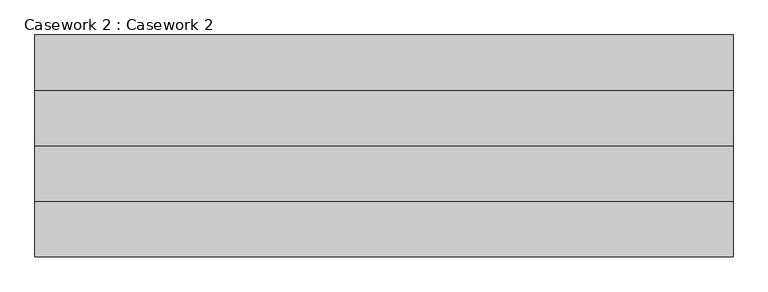
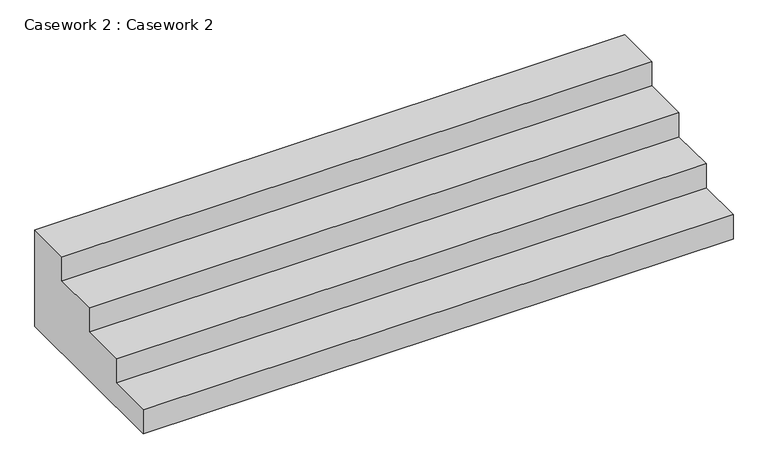
"""IFC4 building model written with IfcOpenShell, lengths in millimetres: furniture geometry, Casework 2 : Casework 2."""

from ifc_helpers import new_model, si_unit, frame, origin, place, context, project, spatial, polyline, outline, extrude, source, transform, mapped, element, save


def casework_2_casework_2_ff1f8355(model_context):
    return source(origin(), model_context, "Body", "SweptSolid", [
        extrude(outline(polyline([(6333.0409313, 457.2), (6333.0409313, 609.6), (6612.4409313, 609.6), (6612.4409313, 0.0), (5494.8409313, 0.0), (5494.8409313, 152.4), (5774.2409313, 152.4), (5774.2409313, 304.8), (6053.6409313, 304.8), (6053.6409313, 457.2), (6333.0409313, 457.2)])), frame((22988.4136801, 0.0, 0.0), z_axis=(1.0, 0.0, 0.0), x_axis=(0.0, 1.0, 0.0)), (0.0, 0.0, 1.0), 3517.9),
    ])


if __name__ == "__main__":
    model = new_model("IFC4")
    model_context = context("Model", 3, world=origin())
    ifc_project = project(units=[si_unit("LENGTHUNIT", "METRE", prefix="MILLI")], contexts=[model_context])
    site = spatial("IfcSite", under=ifc_project)
    building = spatial("IfcBuilding", under=site)
    placement = place(None, origin())
    casework_2_casework_2_shape = casework_2_casework_2_ff1f8355(model_context)
    element("IfcFurniture", 1, ObjectType="Casework 2 : Casework 2", at=placement, inside=building, context=model_context, shape_type="MappedRepresentation", body=[
        mapped(casework_2_casework_2_shape, transform((0.0, 0.0, 0.0), x_axis=(1.0, 0.0, 0.0), y_axis=(0.0, 1.0, 0.0), z_axis=(0.0, 0.0, 1.0))),
    ])
    save(model, "model.ifc")
